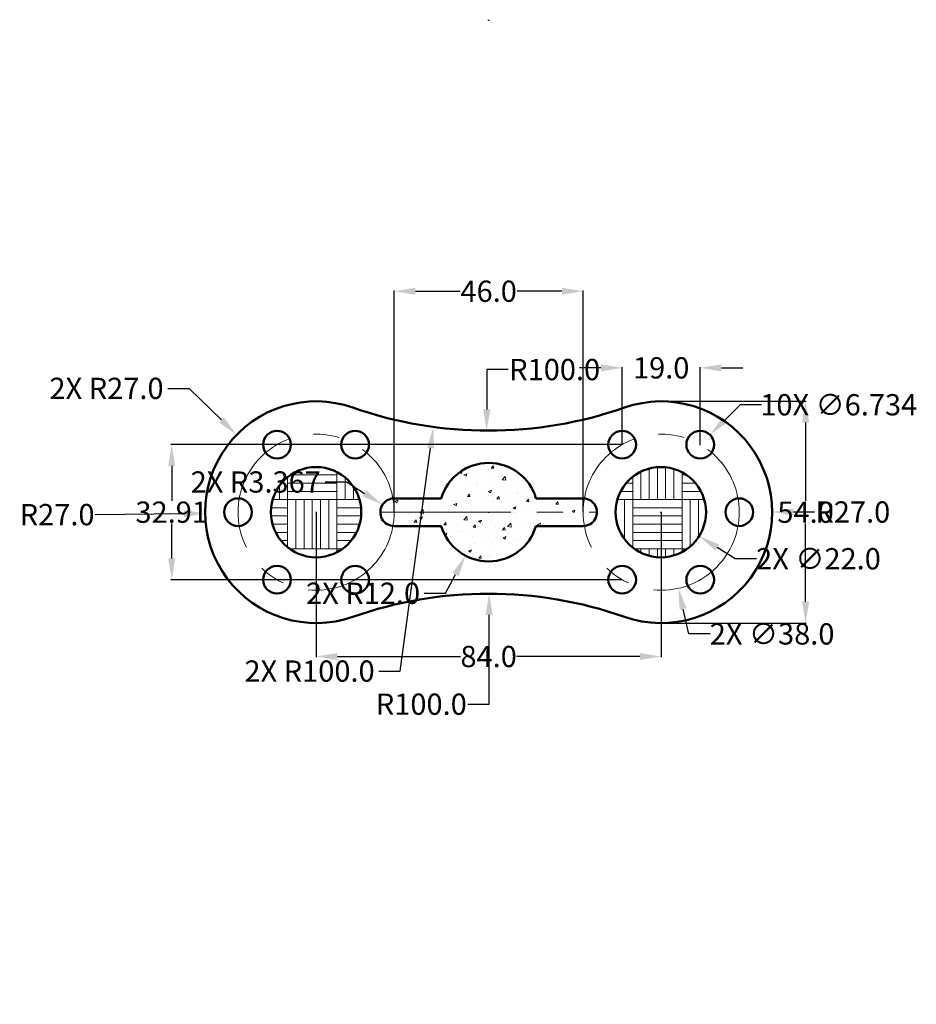
# Model space of a CAD drawing. Units: millimetres. Extents: x 127 to 345, y -63 to 177.
import ezdxf

# ---------------------------------------------------------------- set-up
doc = ezdxf.new("R2010")
doc.units = ezdxf.units.MM
doc.header["$MEASUREMENT"] = 0
doc.linetypes.add('CENTER', pattern=[50.8, 31.75, -6.35, 6.35, -6.35])
for name, color, linetype, lineweight in [('M-CNTR', 4, 'CENTER', 18), ('M-DIMS', 2, 'Continuous', 25), ('M-HATC', 8, 'Continuous', 18), ('M-OUTL', 7, 'Continuous', 50)]:
    doc.layers.add(name, color=color, linetype=linetype, lineweight=lineweight)
doc.styles.get("Standard").update_dxf_attribs({"font": 'arial.ttf'})
doc.dimstyles.get("Standard").update_dxf_attribs({"dimtxt": 5.18, "dimasz": 5.18, "dimexe": 0.18, "dimexo": 0.0625, "dimgap": 0.09, "dimtad": 0, "dimtih": 1, "dimtoh": 1, "dimdec": 1, "dimzin": 0, "dimdsep": 46, "dimtxsty": 'Standard', "dimcen": 0.09, "dimadec": 0, "dimazin": 0, "dimtfac": 1, "dimtdec": 1, "dimtofl": 0, "dimtmove": 0, "dimatfit": 3, "dimfxl": 1, "dimtolj": 1, "dimtzin": 0, "dimarcsym": 0})

# ---------------------------------------------------------------- blocks, each defined once
blk = doc.blocks.new('*D1')
at = {"layer": 'Defpoints', "color": 0, "transparency": 16777216}
for p in [(241.06, 37.08), (240.94, -62.92)]:
    blk.add_point(p, dxfattribs=at)
at = {"layer": 'M-DIMS', "color": 0, "lineweight": -2, "transparency": 16777216}
for p, q in [((241.03, 10.18), (241.06, 31.9)), ((235.85, 10.18), (241.03, 10.18))]:
    blk.add_line(p, q, dxfattribs=at)
at = {"layer": 'M-DIMS', "color": 0, "transparency": 16777216}
blk.add_solid([(240.19, 31.9), (241.92, 31.9), (241.06, 37.08)], dxfattribs=at)
at = {"layer": 'M-DIMS', "color": 0, "transparency": 16777216, "insert": (224.55, 10.18), "char_height": 5.18, "attachment_point": 5}
blk.add_mtext('\\A1;R100.0', dxfattribs=at)
blk = doc.blocks.new('*D2')
at = {"layer": 'Defpoints', "color": 0, "transparency": 16777216}
for p in [(282.94, 56.94), (309.94, 56.97)]:
    blk.add_point(p, dxfattribs=at)
at = {"layer": 'M-DIMS', "color": 0, "lineweight": -2, "transparency": 16777216}
for p, q in [((282.85, 56.94), (283.03, 56.94)), ((282.94, 56.85), (282.94, 57.03)), ((320.3, 56.98), (315.12, 56.97))]:
    blk.add_line(p, q, dxfattribs=at)
at = {"layer": 'M-DIMS', "color": 0, "transparency": 16777216}
blk.add_solid([(315.12, 57.83), (315.12, 56.11), (309.94, 56.97)], dxfattribs=at)
at = {"layer": 'M-DIMS', "color": 0, "transparency": 16777216, "insert": (329.59, 56.98), "char_height": 5.18, "attachment_point": 5}
blk.add_mtext('\\A1;R27.0', dxfattribs=at)
blk = doc.blocks.new('*D3')
at = {"layer": 'Defpoints', "color": 0, "transparency": 16777216}
for p in [(171.94, 56.64), (198.94, 56.94)]:
    blk.add_point(p, dxfattribs=at)
at = {"layer": 'M-DIMS', "color": 0, "lineweight": -2, "transparency": 16777216}
for p, q in [((145.19, 56.34), (166.76, 56.58)), ((198.85, 56.94), (199.03, 56.94)), ((198.94, 56.85), (198.94, 57.03))]:
    blk.add_line(p, q, dxfattribs=at)
at = {"layer": 'M-DIMS', "color": 0, "transparency": 16777216}
blk.add_solid([(166.75, 57.44), (166.77, 55.72), (171.94, 56.64)], dxfattribs=at)
at = {"layer": 'M-DIMS', "color": 0, "transparency": 16777216, "insert": (135.9, 56.34), "char_height": 5.18, "attachment_point": 5}
blk.add_mtext('\\A1;R27.0', dxfattribs=at)
blk = doc.blocks.new('*D4')
at = {"layer": 'Defpoints', "color": 0, "transparency": 16777216}
for p in [(240.94, 176.79), (240.46, 76.79)]:
    blk.add_point(p, dxfattribs=at)
at = {"layer": 'M-DIMS', "color": 0, "lineweight": -2, "transparency": 16777216}
for p, q in [((240.53, 91.67), (240.48, 81.97)), ((245.71, 91.67), (240.53, 91.67))]:
    blk.add_line(p, q, dxfattribs=at)
at = {"layer": 'M-DIMS', "color": 0, "transparency": 16777216}
blk.add_solid([(239.62, 81.98), (241.35, 81.97), (240.46, 76.79)], dxfattribs=at)
at = {"layer": 'M-DIMS', "color": 0, "transparency": 16777216, "insert": (257.01, 91.67), "char_height": 5.18, "attachment_point": 5}
blk.add_mtext('\\A1;R100.0', dxfattribs=at)
blk = doc.blocks.new('*D5')
at = {"layer": 'Defpoints', "color": 0, "transparency": 16777216}
for p in [(263.94, 110.75), (217.94, 56.94), (263.94, 56.94)]:
    blk.add_point(p, dxfattribs=at)
at = {"layer": 'M-DIMS', "color": 0, "lineweight": -2, "transparency": 16777216}
for p, q in [((217.94, 57), (217.94, 110.93)), ((223.12, 110.75), (234.03, 110.75)), ((258.76, 110.75), (247.86, 110.75)), ((263.94, 57), (263.94, 110.93))]:
    blk.add_line(p, q, dxfattribs=at)
at = {"layer": 'M-DIMS', "color": 0, "transparency": 16777216}
for points in [[(223.12, 111.61), (223.12, 109.89), (217.94, 110.75)], [(258.76, 111.61), (258.76, 109.89), (263.94, 110.75)]]:
    blk.add_solid(points, dxfattribs=at)
at = {"layer": 'M-DIMS', "color": 0, "transparency": 16777216, "insert": (240.94, 110.75), "char_height": 5.18, "attachment_point": 5}
blk.add_mtext('\\A1;46.0', dxfattribs=at)
blk = doc.blocks.new('FLANGE-BOLT-PATTERN-5H-PCD38')
for centre in [(-9.5, 16.45), (9.5, 16.45), (-19, 0), (-9.5, -16.45), (9.5, -16.45)]:
    blk.add_circle(centre, 3.37)
blk = doc.blocks.new('*D7')
at = {"layer": 'Defpoints', "color": 0, "transparency": 16777216}
for p in [(198.94, 56.94), (282.94, 56.94), (282.94, 21.79)]:
    blk.add_point(p, dxfattribs=at)
at = {"layer": 'M-DIMS', "color": 0, "lineweight": -2, "transparency": 16777216}
for p, q in [((198.94, 56.87), (198.94, 21.61)), ((282.94, 56.87), (282.94, 21.61)), ((204.12, 21.79), (234.13, 21.79)), ((277.76, 21.79), (247.75, 21.79))]:
    blk.add_line(p, q, dxfattribs=at)
at = {"layer": 'M-DIMS', "color": 0, "transparency": 16777216}
for points in [[(204.12, 22.65), (204.12, 20.93), (198.94, 21.79)], [(277.76, 22.65), (277.76, 20.93), (282.94, 21.79)]]:
    blk.add_solid(points, dxfattribs=at)
at = {"layer": 'M-DIMS', "color": 0, "transparency": 16777216, "insert": (240.94, 21.79), "char_height": 5.18, "attachment_point": 5}
blk.add_mtext('\\A1;84.0', dxfattribs=at)
blk = doc.blocks.new('*D8')
at = {"layer": 'Defpoints', "color": 0, "transparency": 16777216}
for p in [(282.53, 83.94), (318.09, 83.94), (282.53, 29.94)]:
    blk.add_point(p, dxfattribs=at)
at = {"layer": 'M-DIMS', "color": 0, "lineweight": -2, "transparency": 16777216}
for p, q in [((282.59, 83.94), (318.27, 83.94)), ((318.09, 78.76), (318.09, 59.67)), ((318.09, 35.12), (318.09, 54.2)), ((282.59, 29.94), (318.27, 29.94))]:
    blk.add_line(p, q, dxfattribs=at)
at = {"layer": 'M-DIMS', "color": 0, "transparency": 16777216}
for points in [[(317.23, 78.76), (318.96, 78.76), (318.09, 83.94)], [(317.23, 35.12), (318.96, 35.12), (318.09, 29.94)]]:
    blk.add_solid(points, dxfattribs=at)
at = {"layer": 'M-DIMS', "color": 0, "transparency": 16777216, "insert": (318.09, 56.94), "char_height": 5.18, "attachment_point": 5}
blk.add_mtext('\\A1;54.0', dxfattribs=at)
blk = doc.blocks.new('*D9')
at = {"layer": 'Defpoints', "color": 0, "transparency": 16777216}
for p in [(292.44, 92.09), (273.44, 73.39), (292.44, 73.39)]:
    blk.add_point(p, dxfattribs=at)
at = {"layer": 'M-DIMS', "color": 0, "lineweight": -2, "transparency": 16777216}
for p, q in [((268.26, 92.09), (263.08, 92.09)), ((273.44, 73.45), (273.44, 92.27)), ((292.44, 73.45), (292.44, 92.27)), ((297.62, 92.09), (302.8, 92.09))]:
    blk.add_line(p, q, dxfattribs=at)
at = {"layer": 'M-DIMS', "color": 0, "transparency": 16777216}
for points in [[(268.26, 92.95), (268.26, 91.22), (273.44, 92.09)], [(297.62, 92.95), (297.62, 91.22), (292.44, 92.09)]]:
    blk.add_solid(points, dxfattribs=at)
at = {"layer": 'M-DIMS', "color": 0, "transparency": 16777216, "insert": (282.94, 92.09), "char_height": 5.18, "attachment_point": 5}
blk.add_mtext('\\A1;19.0', dxfattribs=at)
blk = doc.blocks.new('*D10')
at = {"layer": 'Defpoints', "color": 0, "transparency": 16777216}
for p in [(163.79, 73.39), (273.44, 73.39), (273.44, 40.48)]:
    blk.add_point(p, dxfattribs=at)
at = {"layer": 'M-DIMS', "color": 0, "lineweight": -2, "transparency": 16777216}
for p, q in [((273.38, 73.39), (163.61, 73.39)), ((163.79, 68.21), (163.79, 59.67)), ((163.79, 45.66), (163.79, 54.2)), ((273.38, 40.48), (163.61, 40.48))]:
    blk.add_line(p, q, dxfattribs=at)
at = {"layer": 'M-DIMS', "color": 0, "transparency": 16777216}
for points in [[(162.93, 68.21), (164.66, 68.21), (163.79, 73.39)], [(162.93, 45.66), (164.66, 45.66), (163.79, 40.48)]]:
    blk.add_solid(points, dxfattribs=at)
at = {"layer": 'M-DIMS', "color": 0, "transparency": 16777216, "insert": (163.79, 56.94), "char_height": 5.18, "attachment_point": 5}
blk.add_mtext('\\A1;32.91', dxfattribs=at)
blk = doc.blocks.new('*D11')
at = {"layer": 'Defpoints', "color": 0, "transparency": 16777216}
for p in [(273.53, 62.78), (292.17, 51.1)]:
    blk.add_point(p, dxfattribs=at)
at = {"layer": 'M-DIMS', "color": 0, "lineweight": -2, "transparency": 16777216}
for p, q in [((282.76, 56.94), (282.94, 56.94)), ((282.85, 56.85), (282.85, 57.03)), ((300.95, 45.6), (296.56, 48.35)), ((306.13, 45.6), (300.95, 45.6))]:
    blk.add_line(p, q, dxfattribs=at)
at = {"layer": 'M-DIMS', "color": 0, "transparency": 16777216}
blk.add_solid([(297.02, 49.08), (296.11, 47.62), (292.17, 51.1)], dxfattribs=at)
at = {"layer": 'M-DIMS', "color": 0, "transparency": 16777216, "insert": (321.23, 45.6), "char_height": 5.18, "attachment_point": 5}
blk.add_mtext('\\A1;2X ∅22.0', dxfattribs=at)
blk = doc.blocks.new('*D12')
at = {"layer": 'Defpoints', "color": 0, "transparency": 16777216}
for p in [(278.74, 75.47), (287.14, 38.41)]:
    blk.add_point(p, dxfattribs=at)
at = {"layer": 'M-DIMS', "color": 0, "lineweight": -2, "transparency": 16777216}
for p, q in [((282.85, 56.94), (283.03, 56.94)), ((282.94, 56.85), (282.94, 57.03)), ((289.66, 27.29), (288.29, 33.35)), ((294.84, 27.29), (289.66, 27.29))]:
    blk.add_line(p, q, dxfattribs=at)
at = {"layer": 'M-DIMS', "color": 0, "transparency": 16777216}
blk.add_solid([(289.13, 33.55), (287.44, 33.16), (287.14, 38.41)], dxfattribs=at)
at = {"layer": 'M-DIMS', "color": 0, "transparency": 16777216, "insert": (309.94, 27.29), "char_height": 5.18, "attachment_point": 5}
blk.add_mtext('\\A1;2X ∅38.0', dxfattribs=at)
blk = doc.blocks.new('*D13')
at = {"layer": 'Defpoints', "color": 0, "transparency": 16777216}
for p in [(179.61, 75.78), (198.94, 56.94)]:
    blk.add_point(p, dxfattribs=at)
at = {"layer": 'M-DIMS', "color": 0, "lineweight": -2, "transparency": 16777216}
for p, q in [((162.83, 87.09), (168.01, 87.09)), ((168.01, 87.09), (175.9, 79.4)), ((198.85, 56.94), (199.03, 56.94)), ((198.94, 56.85), (198.94, 57.03))]:
    blk.add_line(p, q, dxfattribs=at)
at = {"layer": 'M-DIMS', "color": 0, "transparency": 16777216}
blk.add_solid([(176.5, 80.02), (175.3, 78.78), (179.61, 75.78)], dxfattribs=at)
at = {"layer": 'M-DIMS', "color": 0, "transparency": 16777216, "insert": (147.93, 87.09), "char_height": 5.18, "attachment_point": 5}
blk.add_mtext('\\A1;2X R27.0', dxfattribs=at)
blk = doc.blocks.new('*D14')
at = {"layer": 'Defpoints', "color": 0, "transparency": 16777216}
for p in [(240.94, 176.79), (227.5, 77.7)]:
    blk.add_point(p, dxfattribs=at)
at = {"layer": 'M-DIMS', "color": 0, "lineweight": -2, "transparency": 16777216}
for p, q in [((240.85, 176.79), (241.03, 176.79)), ((240.94, 176.7), (240.94, 176.88)), ((219.43, 18.24), (226.8, 72.57)), ((214.25, 18.24), (219.43, 18.24))]:
    blk.add_line(p, q, dxfattribs=at)
at = {"layer": 'M-DIMS', "color": 0, "transparency": 16777216}
blk.add_solid([(225.95, 72.68), (227.66, 72.45), (227.5, 77.7)], dxfattribs=at)
at = {"layer": 'M-DIMS', "color": 0, "transparency": 16777216, "insert": (197.35, 18.24), "char_height": 5.18, "attachment_point": 5}
blk.add_mtext('\\A1;2X R100.0', dxfattribs=at)
blk = doc.blocks.new('*D15')
at = {"layer": 'Defpoints', "color": 0, "transparency": 16777216}
for p in [(294.82, 75.77), (290.06, 71.01)]:
    blk.add_point(p, dxfattribs=at)
at = {"layer": 'M-DIMS', "color": 0, "lineweight": -2, "transparency": 16777216}
for p, q in [((302.15, 83.1), (298.49, 79.44)), ((307.33, 83.1), (302.15, 83.1)), ((292.35, 73.39), (292.53, 73.39)), ((292.44, 73.3), (292.44, 73.48))]:
    blk.add_line(p, q, dxfattribs=at)
at = {"layer": 'M-DIMS', "color": 0, "transparency": 16777216}
blk.add_solid([(297.87, 80.05), (299.1, 78.83), (294.82, 75.77)], dxfattribs=at)
at = {"layer": 'M-DIMS', "color": 0, "transparency": 16777216, "insert": (326.16, 83.1), "char_height": 5.18, "attachment_point": 5}
blk.add_mtext('\\A1;10X ∅6.734', dxfattribs=at)
blk = doc.blocks.new('*D16')
at = {"layer": 'Defpoints', "color": 0, "transparency": 16777216}
for p in [(240.94, 56.94), (235.31, 46.34)]:
    blk.add_point(p, dxfattribs=at)
at = {"layer": 'M-DIMS', "color": 0, "lineweight": -2, "transparency": 16777216}
for p, q in [((240.85, 56.94), (241.03, 56.94)), ((240.94, 56.85), (240.94, 57.03)), ((230.45, 37.19), (232.88, 41.77)), ((225.27, 37.19), (230.45, 37.19))]:
    blk.add_line(p, q, dxfattribs=at)
at = {"layer": 'M-DIMS', "color": 0, "transparency": 16777216}
blk.add_solid([(232.12, 42.17), (233.64, 41.36), (235.31, 46.34)], dxfattribs=at)
at = {"layer": 'M-DIMS', "color": 0, "transparency": 16777216, "insert": (210.37, 37.19), "char_height": 5.18, "attachment_point": 5}
blk.add_mtext('\\A1;2X R12.0', dxfattribs=at)
blk = doc.blocks.new('*D17')
at = {"layer": 'Defpoints', "color": 0, "transparency": 16777216}
for p in [(215.1, 58.74), (217.94, 56.94)]:
    blk.add_point(p, dxfattribs=at)
at = {"layer": 'M-DIMS', "color": 0, "lineweight": -2, "transparency": 16777216}
for p, q in [((201.17, 64.29), (206.35, 64.29)), ((206.35, 64.29), (210.72, 61.51)), ((217.85, 56.94), (218.03, 56.94)), ((217.94, 56.85), (217.94, 57.03))]:
    blk.add_line(p, q, dxfattribs=at)
at = {"layer": 'M-DIMS', "color": 0, "transparency": 16777216}
blk.add_solid([(211.19, 62.24), (210.26, 60.79), (215.1, 58.74)], dxfattribs=at)
at = {"layer": 'M-DIMS', "color": 0, "transparency": 16777216, "insert": (184.25, 64.29), "char_height": 5.18, "attachment_point": 5}
blk.add_mtext('\\A1;2X R3.367', dxfattribs=at)

msp = doc.modelspace()

# ---------------------------------------------------------------- hatches: boundary and pattern name
at = {"layer": 'M-HATC'}
h = msp.add_hatch(dxfattribs=at)
h.set_pattern_fill('AR-PARQ1', color=256)
h.paths.add_polyline_path([(187.9426, 56.9373, 1), (209.9426, 56.9373, 1)])
h.paths.add_polyline_path([(293.8526, 56.9373, 1), (271.8526, 56.9373, 1)])
h = msp.add_hatch(dxfattribs=at)
h.set_pattern_fill('AR-CONC', color=256)
h.paths.add_polyline_path([(263.9426, 56.9373), (217.9426, 56.9373, -0.04438789), (217.6443, 53.5837, 0.02218303), (217.9426, 53.5705), (229.4246, 53.5705, 0.74953576), (252.4606, 53.5705), (263.9426, 53.5705, 0.02218303), (264.2409, 53.5837, -0.04438789)])
h.paths.add_polyline_path([(229.4207, 60.2909), (217.6443, 60.2909, -0.04438789), (217.9426, 56.9373), (263.9426, 56.9373, -0.04438789), (264.2409, 60.2909), (252.4645, 60.2909, 0.75043373)])

# ---------------------------------------------------------------- linework, layer by layer
at = {"layer": 'M-CNTR'}
msp.add_line((214.5757, 56.9373), (267.3094, 56.9373), dxfattribs=at)
for centre in [(198.9426, 56.9373), (282.9426, 56.9373)]:
    msp.add_circle(centre, 19, dxfattribs=at)
at = {"layer": 'M-OUTL'}
for p, q in [((217.6443, 60.2909), (229.4207, 60.2909)), ((264.2409, 60.2909), (252.4645, 60.2909)), ((217.9426, 53.5705), (229.4246, 53.5705)), ((263.9426, 53.5705), (252.4606, 53.5705))]:
    msp.add_line(p, q, dxfattribs=at)
for centre in [(198.9426, 56.9373), (282.8526, 56.9373)]:
    msp.add_circle(centre, 11, dxfattribs=at)
for centre, radius, start, end in [((198.9426, 56.9373), 27, 70.688206, 289.311794), ((282.9426, 56.9373), 27, 250.688206, 109.311794), ((240.9426, 176.7914), 100, 250.688206, 289.311794), ((240.9426, 56.9373), 12, 16.228402, 163.771598), ((217.9426, 56.9373), 3.3668, 84.916859, 270), ((263.9426, 56.9373), 3.3668, 270, 95.083141), ((263.9426, 56.9373), 3.3668, 270, 95.083141), ((240.9426, 56.9373), 12, 196.294259, 343.705741), ((240.9426, -62.9168), 100, 70.688206, 109.311794)]:
    msp.add_arc(centre, radius, start, end, dxfattribs=at)

# ---------------------------------------------------------------- block references
msp.add_blockref('FLANGE-BOLT-PATTERN-5H-PCD38', (198.9426, 56.9373), dxfattribs=at)
at = {"layer": 'M-OUTL', "rotation": 180}
msp.add_blockref('FLANGE-BOLT-PATTERN-5H-PCD38', (282.9426, 56.9373), dxfattribs=at)

# ---------------------------------------------------------------- dimensions: what is measured, and where the dimension line sits
at = {"layer": 'M-DIMS'}
for center, mpoint, picture, middle in [((240.9426, 176.7914), (227.4999, 77.699), '*D14', (197.3451, 18.2436)), ((198.9426, 56.9373), (179.6073, 75.7826), '*D13', (147.9293, 87.0898))]:
    dim = msp.add_radius_dim(center=center, mpoint=mpoint, text='2X <>', dimstyle='Standard', override={"dimdec": 1, "dimlfac": 1, "dimrnd": 0, "dimzin": 0, "dimdsep": 46, "dimlunit": 2}, dxfattribs=at)
    dim.commit()
    dim.dimension.update_dxf_attribs({"geometry": picture, "text_midpoint": middle, "dimtype": 164})
for center, mpoint, picture, middle in [((240.9426, 176.7914), (240.459, 76.7926), '*D4', (257.0107, 91.665)), ((198.9426, 56.9373), (171.9443, 56.6374), '*D3', (145.1893, 56.3401)), ((240.9426, -62.9168), (241.0634, 37.0832), '*D1', (224.5511, 10.1776))]:
    dim = msp.add_radius_dim(center=center, mpoint=mpoint, dimstyle='Standard', override={"dimclrd": 0, "dimclre": 0, "dimclrt": 0}, dxfattribs=at)
    dim.commit()
    dim.dimension.update_dxf_attribs({"geometry": picture, "text_midpoint": middle, "dimtype": 164})
for base, p1, p2, override, picture, middle in [((263.9426, 110.7487), (217.9426, 56.9373), (263.9426, 56.9373), {"dimclrd": 0, "dimclre": 0, "dimclrt": 0}, '*D5', (240.9426, 110.7487)), ((292.4426, 92.0861), (273.4426, 73.3918), (292.4426, 73.3918), {"dimdec": 1, "dimlfac": 1, "dimrnd": 0, "dimzin": 0, "dimdsep": 46, "dimlunit": 2}, '*D9', (282.9426, 92.0861)), ((282.9426, 21.7885), (198.9426, 56.9373), (282.9426, 56.9373), {"dimdec": 1, "dimlfac": 1, "dimrnd": 0, "dimzin": 0, "dimdsep": 46, "dimlunit": 2}, '*D7', (240.9426, 21.7885))]:
    dim = msp.add_linear_dim(base=base, p1=p1, p2=p2, dimstyle='Standard', override=override, dxfattribs=at)
    dim.commit()
    dim.dimension.update_dxf_attribs({"geometry": picture, "text_midpoint": middle})
for p1, p2, text, override, picture, middle in [((290.0623, 71.0107), (294.8229, 75.7729), '10X <>', {"dimdec": 3, "dimlfac": 1, "dimrnd": 0, "dimzin": 0, "dimdsep": 46, "dimlunit": 2}, '*D15', (326.1604, 83.0998)), ((278.7445, 75.4677), (287.1407, 38.4069), '2X <>', {"dimdec": 1, "dimlfac": 1, "dimrnd": 0, "dimzin": 0, "dimdsep": 46, "dimlunit": 2}, '*D12', (309.9378, 27.2887)), ((273.5308, 62.7772), (292.1744, 51.0974), '2X <>', {"dimdec": 1, "dimlfac": 1, "dimrnd": 0, "dimzin": 0, "dimdsep": 46, "dimlunit": 2}, '*D11', (321.232, 45.5972))]:
    dim = msp.add_diameter_dim_2p(p1=p1, p2=p2, text=text, dimstyle='Standard', override=override, dxfattribs=at)
    dim.commit()
    dim.dimension.update_dxf_attribs({"geometry": picture, "text_midpoint": middle, "dimtype": 163})
for base, p1, p2, override, picture, middle in [((318.0926, 83.9361), (282.5306, 29.9385), (282.5306, 83.9361), {"dimdec": 1, "dimlfac": 1, "dimrnd": 0, "dimzin": 0, "dimdsep": 46, "dimlunit": 2}, '*D8', (318.0926, 56.9373)), ((163.7926, 73.3918), (273.4426, 40.4828), (273.4426, 73.3918), {"dimdec": 2, "dimlfac": 1, "dimrnd": 0, "dimzin": 0, "dimdsep": 46, "dimlunit": 2}, '*D10', (163.7926, 56.9373))]:
    dim = msp.add_linear_dim(base=base, p1=p1, p2=p2, angle=90, dimstyle='Standard', override=override, dxfattribs=at)
    dim.commit()
    dim.dimension.update_dxf_attribs({"geometry": picture, "text_midpoint": middle})
for center, mpoint, override, picture, middle in [((217.9426, 56.9373), (215.0993, 58.7404), {"dimdec": 3, "dimlfac": 1, "dimrnd": 0, "dimzin": 0, "dimdsep": 46, "dimlunit": 2}, '*D17', (184.2523, 64.2888)), ((240.9426, 56.9373), (235.3106, 46.3411), {"dimdec": 1, "dimlfac": 1, "dimrnd": 0, "dimzin": 0, "dimdsep": 46, "dimlunit": 2}, '*D16', (210.3714, 37.193))]:
    dim = msp.add_radius_dim(center=center, mpoint=mpoint, text='2X <>', dimstyle='Standard', override=override, dxfattribs=at)
    dim.commit()
    dim.dimension.update_dxf_attribs({"geometry": picture, "text_midpoint": middle})
dim = msp.add_radius_dim(center=(282.9426, 56.9373), mpoint=(309.9426, 56.9655), dimstyle='Standard', override={"dimclrd": 0, "dimclre": 0, "dimclrt": 0}, dxfattribs=at)
dim.commit()
dim.dimension.update_dxf_attribs({"geometry": '*D2', "text_midpoint": (329.5901, 56.9763)})

doc.saveas('drawing.dxf')
